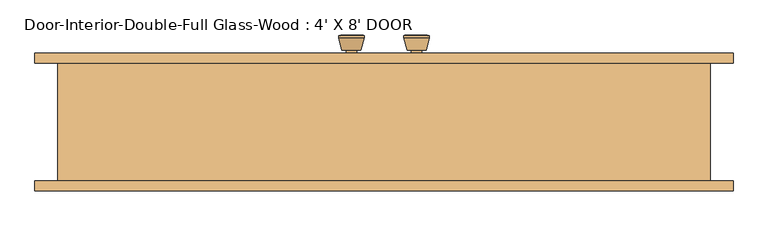
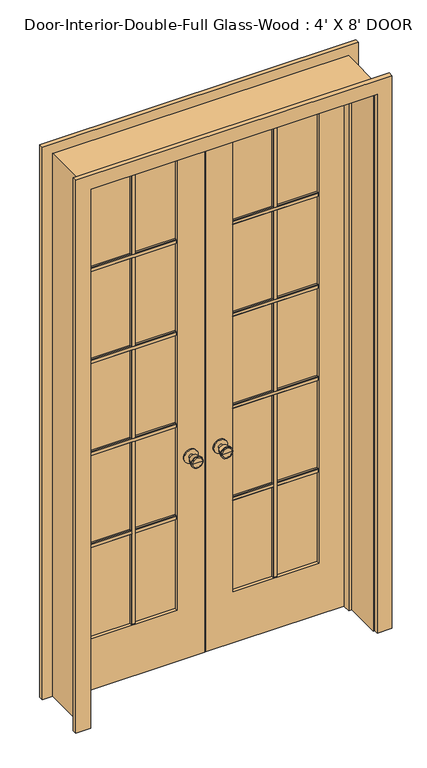
"""IFC4 building model written with IfcOpenShell, lengths in millimetres: door geometry, Door-Interior-Double-Full Glass-Wood : 4' X 8' DOOR."""

from ifc_helpers import new_model, si_unit, point, frame, frame_2d, origin, place, context, project, spatial, polyline, circle_curve, trimmed, segment, composite_curve, outline, extrude, faceted_brep, source, transform, mapped, element, save
from ifc_brep_helpers import plane_surface, cylinder_surface, revolved_surface, advanced_brep


def door_interior_double_full_glass_wood_4_x_8_door_7870f6d1(model_context):
    return source(origin(), model_context, "Body", "SolidModel", [
        advanced_brep(
        [(-63.5, 117.825, 914.4), (-73.5, 117.825, 914.4), (-53.5, 117.825, 914.4), (-83.9758676, 166.825, 914.4), (-63.5, 166.825, 914.4), (-43.0241324, 166.825, 914.4), (-88.5, 164.9971319, 914.4), (-38.5, 164.9971319, 914.4), (-88.5, 161.5334537, 914.4), (-38.5, 161.5334537, 914.4), (-82.136236, 136.825, 914.4), (-44.863764, 136.825, 914.4), (-73.5, 136.825, 914.4), (-53.5, 136.825, 914.4)],
        [
            (0, 1),
            (1, 2, circle_curve(frame((-63.5, 117.825, 914.4), z_axis=(0.0, -1.0, 0.0), x_axis=(1.0, 0.0, 0.0)), 10.0)),
            (2, 0),
            (2, 1, circle_curve(frame((-63.5, 117.825, 914.4), z_axis=(0.0, -1.0, 0.0), x_axis=(1.0, 0.0, 0.0)), 10.0)),
            (3, 4),
            (4, 5),
            (5, 3, circle_curve(frame((-63.5, 166.825, 914.4), z_axis=(0.0, 1.0, 0.0), x_axis=(1.0, 0.0, 0.0)), 20.4758676)),
            (3, 5, circle_curve(frame((-63.5, 166.825, 914.4), z_axis=(0.0, 1.0, 0.0), x_axis=(1.0, 0.0, 0.0)), 20.4758676)),
            (6, 3),
            (5, 7),
            (7, 6, circle_curve(frame((-63.5, 164.9971319, 914.4), z_axis=(0.0, 1.0, 0.0), x_axis=(1.0, 0.0, 0.0)), 25.0)),
            (6, 7, circle_curve(frame((-63.5, 164.9971319, 914.4), z_axis=(0.0, 1.0, 0.0), x_axis=(1.0, 0.0, 0.0)), 25.0)),
            (8, 6),
            (7, 9),
            (9, 8, circle_curve(frame((-63.5, 161.5334537, 914.4), z_axis=(0.0, 1.0, 0.0), x_axis=(1.0, 0.0, 0.0)), 25.0)),
            (8, 9, circle_curve(frame((-63.5, 161.5334537, 914.4), z_axis=(0.0, 1.0, 0.0), x_axis=(1.0, 0.0, 0.0)), 25.0)),
            (10, 8),
            (9, 11),
            (11, 10, circle_curve(frame((-63.5, 136.825, 914.4), z_axis=(0.0, 1.0, 0.0), x_axis=(1.0, 0.0, 0.0)), 18.636236)),
            (10, 11, circle_curve(frame((-63.5, 136.825, 914.4), z_axis=(0.0, 1.0, 0.0), x_axis=(1.0, 0.0, 0.0)), 18.636236)),
            (12, 10),
            (11, 13),
            (13, 12, circle_curve(frame((-63.5, 136.825, 914.4), z_axis=(0.0, 1.0, 0.0), x_axis=(1.0, 0.0, 0.0)), 10.0)),
            (12, 13, circle_curve(frame((-63.5, 136.825, 914.4), z_axis=(0.0, 1.0, 0.0), x_axis=(1.0, 0.0, 0.0)), 10.0)),
            (1, 12),
            (13, 2),
        ],
        [
            plane_surface(frame((-63.5, 117.825, 914.4), z_axis=(0.0, -1.0, 0.0), x_axis=(1.0, 0.0, 0.0))),
            plane_surface(frame((-63.5, 166.825, 914.4), z_axis=(0.0, 1.0, 0.0), x_axis=(1.0, 0.0, 0.0))),
            revolved_surface(polyline([(-43.0241324, 166.825, 914.4), (-38.5, 164.9971319, 914.4)]), (-63.5, 117.825, 914.4), (0.0, -1.0, 0.0)),
            cylinder_surface(frame((-63.5, 117.825, 914.4), z_axis=(0.0, -1.0, 0.0), x_axis=(1.0, 0.0, 0.0)), 25.0),
            revolved_surface(polyline([(-38.5, 161.5334537, 914.4), (-44.863764, 136.825, 914.4)]), (-63.5, 117.825, 914.4), (0.0, -1.0, 0.0)),
            plane_surface(frame((-63.5, 136.825, 914.4), z_axis=(0.0, -1.0, 0.0), x_axis=(1.0, 0.0, 0.0))),
            cylinder_surface(frame((-63.5, 117.825, 914.4), z_axis=(0.0, -1.0, 0.0), x_axis=(1.0, 0.0, 0.0)), 10.0),
        ],
        [
            (0, [[1, 2, 3]]),
            (0, [[-3, 4, -1]]),
            (1, [[5, 6, 7]]),
            (1, [[-6, -5, 8]]),
            (2, [[9, -7, 10, 11]]),
            (2, [[-10, -8, -9, 12]]),
            (3, [[13, -11, 14, 15]]),
            (3, [[-14, -12, -13, 16]]),
            (4, [[17, -15, 18, 19]]),
            (4, [[-18, -16, -17, 20]]),
            (5, [[21, -19, 22, 23]]),
            (5, [[-22, -20, -21, 24]]),
            (6, [[25, -23, 26, -2]]),
            (6, [[-26, -24, -25, -4]]),
        ],
    ),
        extrude(outline(composite_curve([segment(trimmed(circle_curve(frame_2d((914.4, -63.5)), 30.0), [point((914.4, -33.5))], [point((914.4, -93.5))], False, "CARTESIAN"), True, "CONTINUOUS"), segment(trimmed(circle_curve(frame_2d((914.4, -63.5)), 30.0), [point((914.4, -93.5))], [point((914.4, -33.5))], False, "CARTESIAN"), True, "CONTINUOUS")], self_intersect=False)), frame((0.0, 111.825, 0.0), z_axis=(0.0, 1.0, 0.0), x_axis=(0.0, 0.0, 1.0)), (0.0, 0.0, 1.0), 6.0),
        advanced_brep(
        [(-63.5, 70.9, 914.4), (-53.5, 70.9, 914.4), (-73.5, 70.9, 914.4), (-83.9758676, 21.9, 914.4), (-43.0241324, 21.9, 914.4), (-63.5, 21.9, 914.4), (-88.5, 23.7278681, 914.4), (-38.5, 23.7278681, 914.4), (-88.5, 27.1915463, 914.4), (-38.5, 27.1915463, 914.4), (-82.136236, 51.9, 914.4), (-44.863764, 51.9, 914.4), (-73.5, 51.9, 914.4), (-53.5, 51.9, 914.4)],
        [
            (0, 1),
            (1, 2, circle_curve(frame((-63.5, 70.9, 914.4), z_axis=(0.0, 1.0, 0.0), x_axis=(1.0, 0.0, 0.0)), 10.0)),
            (2, 0),
            (2, 1, circle_curve(frame((-63.5, 70.9, 914.4), z_axis=(0.0, 1.0, 0.0), x_axis=(1.0, 0.0, 0.0)), 10.0)),
            (3, 4, circle_curve(frame((-63.5, 21.9, 914.4), z_axis=(0.0, -1.0, 0.0), x_axis=(1.0, 0.0, 0.0)), 20.4758676)),
            (4, 5),
            (5, 3),
            (4, 3, circle_curve(frame((-63.5, 21.9, 914.4), z_axis=(0.0, -1.0, 0.0), x_axis=(1.0, 0.0, 0.0)), 20.4758676)),
            (6, 7, circle_curve(frame((-63.5, 23.7278681, 914.4), z_axis=(0.0, -1.0, 0.0), x_axis=(1.0, 0.0, 0.0)), 25.0)),
            (7, 4),
            (3, 6),
            (7, 6, circle_curve(frame((-63.5, 23.7278681, 914.4), z_axis=(0.0, -1.0, 0.0), x_axis=(1.0, 0.0, 0.0)), 25.0)),
            (8, 9, circle_curve(frame((-63.5, 27.1915463, 914.4), z_axis=(0.0, -1.0, 0.0), x_axis=(1.0, 0.0, 0.0)), 25.0)),
            (9, 7),
            (6, 8),
            (9, 8, circle_curve(frame((-63.5, 27.1915463, 914.4), z_axis=(0.0, -1.0, 0.0), x_axis=(1.0, 0.0, 0.0)), 25.0)),
            (10, 11, circle_curve(frame((-63.5, 51.9, 914.4), z_axis=(0.0, -1.0, 0.0), x_axis=(1.0, 0.0, 0.0)), 18.636236)),
            (11, 9),
            (8, 10),
            (11, 10, circle_curve(frame((-63.5, 51.9, 914.4), z_axis=(0.0, -1.0, 0.0), x_axis=(1.0, 0.0, 0.0)), 18.636236)),
            (12, 13, circle_curve(frame((-63.5, 51.9, 914.4), z_axis=(0.0, -1.0, 0.0), x_axis=(1.0, 0.0, 0.0)), 10.0)),
            (13, 11),
            (10, 12),
            (13, 12, circle_curve(frame((-63.5, 51.9, 914.4), z_axis=(0.0, -1.0, 0.0), x_axis=(1.0, 0.0, 0.0)), 10.0)),
            (1, 13),
            (12, 2),
        ],
        [
            plane_surface(frame((-63.5, 70.9, 914.4), z_axis=(0.0, 1.0, 0.0), x_axis=(1.0, 0.0, 0.0))),
            plane_surface(frame((-63.5, 21.9, 914.4), z_axis=(0.0, -1.0, 0.0), x_axis=(1.0, 0.0, 0.0))),
            revolved_surface(polyline([(-43.0241324, 21.9, 914.4), (-38.5, 23.7278681, 914.4)]), (-63.5, 70.9, 914.4), (0.0, 1.0, 0.0)),
            cylinder_surface(frame((-63.5, 70.9, 914.4), z_axis=(0.0, 1.0, 0.0), x_axis=(1.0, 0.0, 0.0)), 25.0),
            revolved_surface(polyline([(-38.5, 27.1915463, 914.4), (-44.863764, 51.9, 914.4)]), (-63.5, 70.9, 914.4), (0.0, 1.0, 0.0)),
            plane_surface(frame((-63.5, 51.9, 914.4), z_axis=(0.0, 1.0, 0.0), x_axis=(1.0, 0.0, 0.0))),
            cylinder_surface(frame((-63.5, 70.9, 914.4), z_axis=(0.0, 1.0, 0.0), x_axis=(1.0, 0.0, 0.0)), 10.0),
        ],
        [
            (0, [[1, 2, 3]]),
            (0, [[-3, 4, -1]]),
            (1, [[5, 6, 7]]),
            (1, [[8, -7, -6]]),
            (2, [[9, 10, -5, 11]]),
            (2, [[12, -11, -8, -10]]),
            (3, [[13, 14, -9, 15]]),
            (3, [[16, -15, -12, -14]]),
            (4, [[17, 18, -13, 19]]),
            (4, [[20, -19, -16, -18]]),
            (5, [[21, 22, -17, 23]]),
            (5, [[24, -23, -20, -22]]),
            (6, [[-2, 25, -21, 26]]),
            (6, [[-4, -26, -24, -25]]),
        ],
    ),
        extrude(outline(composite_curve([segment(trimmed(circle_curve(frame_2d((914.4, -63.5)), 30.0), [point((914.4, -33.5))], [point((914.4, -93.5))], False, "CARTESIAN"), True, "CONTINUOUS"), segment(trimmed(circle_curve(frame_2d((914.4, -63.5)), 30.0), [point((914.4, -93.5))], [point((914.4, -33.5))], False, "CARTESIAN"), True, "CONTINUOUS")], self_intersect=False)), frame((0.0, 70.9, 0.0), z_axis=(0.0, 1.0, 0.0), x_axis=(0.0, 0.0, 1.0)), (0.0, 0.0, 1.0), 6.0),
        extrude(outline(polyline([(90.87, 1911.35), (90.87, 1892.3), (84.52, 1892.3), (81.345, 1895.475), (81.345, 1908.175), (84.52, 1911.35), (90.87, 1911.35)])), frame((120.65, 0.0, 0.0), z_axis=(1.0, 0.0, 0.0), x_axis=(0.0, 1.0, 0.0)), (0.0, 0.0, 1.0), 368.3),
        extrude(outline(polyline([(90.87, 1493.8375), (90.87, 1474.7875), (84.52, 1474.7875), (81.345, 1477.9625), (81.345, 1490.6625), (84.52, 1493.8375), (90.87, 1493.8375)])), frame((120.65, 0.0, 0.0), z_axis=(1.0, 0.0, 0.0), x_axis=(0.0, 1.0, 0.0)), (0.0, 0.0, 1.0), 368.3),
        extrude(outline(polyline([(90.87, 1076.325), (90.87, 1057.275), (84.52, 1057.275), (81.345, 1060.45), (81.345, 1073.15), (84.52, 1076.325), (90.87, 1076.325)])), frame((120.65, 0.0, 0.0), z_axis=(1.0, 0.0, 0.0), x_axis=(0.0, 1.0, 0.0)), (0.0, 0.0, 1.0), 368.3),
        extrude(outline(polyline([(295.275, 90.87), (314.325, 90.87), (314.325, 84.52), (311.15, 81.345), (298.45, 81.345), (295.275, 84.52), (295.275, 90.87)])), frame((0.0, 0.0, 231.775), z_axis=(0.0, 0.0, 1.0), x_axis=(1.0, 0.0, 0.0)), (0.0, 0.0, 1.0), 2087.5625),
        extrude(outline(polyline([(90.87, 658.8125), (90.87, 639.7625), (84.52, 639.7625), (81.345, 642.9375), (81.345, 655.6375), (84.52, 658.8125), (90.87, 658.8125)])), frame((120.65, 0.0, 0.0), z_axis=(1.0, 0.0, 0.0), x_axis=(0.0, 1.0, 0.0)), (0.0, 0.0, 1.0), 368.3),
        extrude(outline(polyline([(97.855, 1911.35), (104.205, 1911.35), (107.38, 1908.175), (107.38, 1895.475), (104.205, 1892.3), (97.855, 1892.3), (97.855, 1911.35)])), frame((-488.95, 0.0, 0.0), z_axis=(1.0, 0.0, 0.0), x_axis=(0.0, 1.0, 0.0)), (0.0, 0.0, 1.0), 368.3),
        extrude(outline(polyline([(97.855, 1493.8375), (104.205, 1493.8375), (107.38, 1490.6625), (107.38, 1477.9625), (104.205, 1474.7875), (97.855, 1474.7875), (97.855, 1493.8375)])), frame((-488.95, 0.0, 0.0), z_axis=(1.0, 0.0, 0.0), x_axis=(0.0, 1.0, 0.0)), (0.0, 0.0, 1.0), 368.3),
        extrude(outline(polyline([(97.855, 1076.325), (104.205, 1076.325), (107.38, 1073.15), (107.38, 1060.45), (104.205, 1057.275), (97.855, 1057.275), (97.855, 1076.325)])), frame((-488.95, 0.0, 0.0), z_axis=(1.0, 0.0, 0.0), x_axis=(0.0, 1.0, 0.0)), (0.0, 0.0, 1.0), 368.3),
        extrude(outline(polyline([(-314.325, 97.855), (-314.325, 104.205), (-311.15, 107.38), (-298.45, 107.38), (-295.275, 104.205), (-295.275, 97.855), (-314.325, 97.855)])), frame((0.0, 0.0, 231.775), z_axis=(0.0, 0.0, 1.0), x_axis=(1.0, 0.0, 0.0)), (0.0, 0.0, 1.0), 2087.5625),
        extrude(outline(polyline([(97.855, 658.8125), (104.205, 658.8125), (107.38, 655.6375), (107.38, 642.9375), (104.205, 639.7625), (97.855, 639.7625), (97.855, 658.8125)])), frame((-488.95, 0.0, 0.0), z_axis=(1.0, 0.0, 0.0), x_axis=(0.0, 1.0, 0.0)), (0.0, 0.0, 1.0), 368.3),
        extrude(outline(polyline([(97.855, 1911.35), (104.205, 1911.35), (107.38, 1908.175), (107.38, 1895.475), (104.205, 1892.3), (97.855, 1892.3), (97.855, 1911.35)])), frame((120.65, 0.0, 0.0), z_axis=(1.0, 0.0, 0.0), x_axis=(0.0, 1.0, 0.0)), (0.0, 0.0, 1.0), 368.3),
        extrude(outline(polyline([(97.855, 1493.8375), (104.205, 1493.8375), (107.38, 1490.6625), (107.38, 1477.9625), (104.205, 1474.7875), (97.855, 1474.7875), (97.855, 1493.8375)])), frame((120.65, 0.0, 0.0), z_axis=(1.0, 0.0, 0.0), x_axis=(0.0, 1.0, 0.0)), (0.0, 0.0, 1.0), 368.3),
        extrude(outline(polyline([(97.855, 1076.325), (104.205, 1076.325), (107.38, 1073.15), (107.38, 1060.45), (104.205, 1057.275), (97.855, 1057.275), (97.855, 1076.325)])), frame((120.65, 0.0, 0.0), z_axis=(1.0, 0.0, 0.0), x_axis=(0.0, 1.0, 0.0)), (0.0, 0.0, 1.0), 368.3),
        extrude(outline(polyline([(295.275, 97.855), (295.275, 104.205), (298.45, 107.38), (311.15, 107.38), (314.325, 104.205), (314.325, 97.855), (295.275, 97.855)])), frame((0.0, 0.0, 231.775), z_axis=(0.0, 0.0, 1.0), x_axis=(1.0, 0.0, 0.0)), (0.0, 0.0, 1.0), 2087.5625),
        extrude(outline(polyline([(97.855, 658.8125), (104.205, 658.8125), (107.38, 655.6375), (107.38, 642.9375), (104.205, 639.7625), (97.855, 639.7625), (97.855, 658.8125)])), frame((120.65, 0.0, 0.0), z_axis=(1.0, 0.0, 0.0), x_axis=(0.0, 1.0, 0.0)), (0.0, 0.0, 1.0), 368.3),
        extrude(outline(polyline([(90.87, 1911.35), (90.87, 1892.3), (84.52, 1892.3), (81.345, 1895.475), (81.345, 1908.175), (84.52, 1911.35), (90.87, 1911.35)])), frame((-488.95, 0.0, 0.0), z_axis=(1.0, 0.0, 0.0), x_axis=(0.0, 1.0, 0.0)), (0.0, 0.0, 1.0), 368.3),
        extrude(outline(polyline([(90.87, 1493.8375), (90.87, 1474.7875), (84.52, 1474.7875), (81.345, 1477.9625), (81.345, 1490.6625), (84.52, 1493.8375), (90.87, 1493.8375)])), frame((-488.95, 0.0, 0.0), z_axis=(1.0, 0.0, 0.0), x_axis=(0.0, 1.0, 0.0)), (0.0, 0.0, 1.0), 368.3),
        extrude(outline(polyline([(90.87, 1076.325), (90.87, 1057.275), (84.52, 1057.275), (81.345, 1060.45), (81.345, 1073.15), (84.52, 1076.325), (90.87, 1076.325)])), frame((-488.95, 0.0, 0.0), z_axis=(1.0, 0.0, 0.0), x_axis=(0.0, 1.0, 0.0)), (0.0, 0.0, 1.0), 368.3),
        extrude(outline(polyline([(-314.325, 90.87), (-295.275, 90.87), (-295.275, 84.52), (-298.45, 81.345), (-311.15, 81.345), (-314.325, 84.52), (-314.325, 90.87)])), frame((0.0, 0.0, 231.775), z_axis=(0.0, 0.0, 1.0), x_axis=(1.0, 0.0, 0.0)), (0.0, 0.0, 1.0), 2087.5625),
        extrude(outline(polyline([(90.87, 658.8125), (90.87, 639.7625), (84.52, 639.7625), (81.345, 642.9375), (81.345, 655.6375), (84.52, 658.8125), (90.87, 658.8125)])), frame((-488.95, 0.0, 0.0), z_axis=(1.0, 0.0, 0.0), x_axis=(0.0, 1.0, 0.0)), (0.0, 0.0, 1.0), 368.3),
        advanced_brep(
        [(63.5, 70.9, 914.4), (73.5, 70.9, 914.4), (53.5, 70.9, 914.4), (83.9758676, 21.9, 914.4), (63.5, 21.9, 914.4), (43.0241324, 21.9, 914.4), (88.5, 23.7278681, 914.4), (38.5, 23.7278681, 914.4), (88.5, 27.1915463, 914.4), (38.5, 27.1915463, 914.4), (82.136236, 51.9, 914.4), (44.863764, 51.9, 914.4), (73.5, 51.9, 914.4), (53.5, 51.9, 914.4)],
        [
            (0, 1),
            (1, 2, circle_curve(frame((63.5, 70.9, 914.4), z_axis=(0.0, 1.0, 0.0), x_axis=(-1.0, 0.0, 0.0)), 10.0)),
            (2, 0),
            (2, 1, circle_curve(frame((63.5, 70.9, 914.4), z_axis=(0.0, 1.0, 0.0), x_axis=(-1.0, 0.0, 0.0)), 10.0)),
            (3, 4),
            (4, 5),
            (5, 3, circle_curve(frame((63.5, 21.9, 914.4), z_axis=(0.0, -1.0, 0.0), x_axis=(-1.0, 0.0, 0.0)), 20.4758676)),
            (3, 5, circle_curve(frame((63.5, 21.9, 914.4), z_axis=(0.0, -1.0, 0.0), x_axis=(-1.0, 0.0, 0.0)), 20.4758676)),
            (6, 3),
            (5, 7),
            (7, 6, circle_curve(frame((63.5, 23.7278681, 914.4), z_axis=(0.0, -1.0, 0.0), x_axis=(-1.0, 0.0, 0.0)), 25.0)),
            (6, 7, circle_curve(frame((63.5, 23.7278681, 914.4), z_axis=(0.0, -1.0, 0.0), x_axis=(-1.0, 0.0, 0.0)), 25.0)),
            (8, 6),
            (7, 9),
            (9, 8, circle_curve(frame((63.5, 27.1915463, 914.4), z_axis=(0.0, -1.0, 0.0), x_axis=(-1.0, 0.0, 0.0)), 25.0)),
            (8, 9, circle_curve(frame((63.5, 27.1915463, 914.4), z_axis=(0.0, -1.0, 0.0), x_axis=(-1.0, 0.0, 0.0)), 25.0)),
            (10, 8),
            (9, 11),
            (11, 10, circle_curve(frame((63.5, 51.9, 914.4), z_axis=(0.0, -1.0, 0.0), x_axis=(-1.0, 0.0, 0.0)), 18.636236)),
            (10, 11, circle_curve(frame((63.5, 51.9, 914.4), z_axis=(0.0, -1.0, 0.0), x_axis=(-1.0, 0.0, 0.0)), 18.636236)),
            (12, 10),
            (11, 13),
            (13, 12, circle_curve(frame((63.5, 51.9, 914.4), z_axis=(0.0, -1.0, 0.0), x_axis=(-1.0, 0.0, 0.0)), 10.0)),
            (12, 13, circle_curve(frame((63.5, 51.9, 914.4), z_axis=(0.0, -1.0, 0.0), x_axis=(-1.0, 0.0, 0.0)), 10.0)),
            (1, 12),
            (13, 2),
        ],
        [
            plane_surface(frame((63.5, 70.9, 914.4), z_axis=(0.0, 1.0, 0.0), x_axis=(-1.0, 0.0, 0.0))),
            plane_surface(frame((63.5, 21.9, 914.4), z_axis=(0.0, -1.0, 0.0), x_axis=(-1.0, 0.0, 0.0))),
            revolved_surface(polyline([(43.0241324, 21.9, 914.4), (38.5, 23.7278681, 914.4)]), (63.5, 70.9, 914.4), (0.0, 1.0, 0.0)),
            cylinder_surface(frame((63.5, 70.9, 914.4), z_axis=(0.0, 1.0, 0.0), x_axis=(-1.0, 0.0, 0.0)), 25.0),
            revolved_surface(polyline([(38.5, 27.1915463, 914.4), (44.863764, 51.9, 914.4)]), (63.5, 70.9, 914.4), (0.0, 1.0, 0.0)),
            plane_surface(frame((63.5, 51.9, 914.4), z_axis=(0.0, 1.0, 0.0), x_axis=(-1.0, 0.0, 0.0))),
            cylinder_surface(frame((63.5, 70.9, 914.4), z_axis=(0.0, 1.0, 0.0), x_axis=(-1.0, 0.0, 0.0)), 10.0),
        ],
        [
            (0, [[1, 2, 3]]),
            (0, [[-3, 4, -1]]),
            (1, [[5, 6, 7]]),
            (1, [[-6, -5, 8]]),
            (2, [[9, -7, 10, 11]]),
            (2, [[-10, -8, -9, 12]]),
            (3, [[13, -11, 14, 15]]),
            (3, [[-14, -12, -13, 16]]),
            (4, [[17, -15, 18, 19]]),
            (4, [[-18, -16, -17, 20]]),
            (5, [[21, -19, 22, 23]]),
            (5, [[-22, -20, -21, 24]]),
            (6, [[25, -23, 26, -2]]),
            (6, [[-26, -24, -25, -4]]),
        ],
    ),
        extrude(outline(composite_curve([segment(trimmed(circle_curve(frame_2d((914.4, 63.5)), 30.0), [point((914.4, 33.5))], [point((914.4, 93.5))], False, "CARTESIAN"), True, "CONTINUOUS"), segment(trimmed(circle_curve(frame_2d((914.4, 63.5)), 30.0), [point((914.4, 93.5))], [point((914.4, 33.5))], False, "CARTESIAN"), True, "CONTINUOUS")], self_intersect=False)), frame((0.0, 70.9, 0.0), z_axis=(0.0, 1.0, 0.0), x_axis=(0.0, 0.0, 1.0)), (0.0, 0.0, 1.0), 6.0),
        advanced_brep(
        [(63.5, 117.825, 914.4), (53.5, 117.825, 914.4), (73.5, 117.825, 914.4), (83.9758676, 166.825, 914.4), (43.0241324, 166.825, 914.4), (63.5, 166.825, 914.4), (88.5, 164.9971319, 914.4), (38.5, 164.9971319, 914.4), (88.5, 161.5334537, 914.4), (38.5, 161.5334537, 914.4), (82.136236, 136.825, 914.4), (44.863764, 136.825, 914.4), (73.5, 136.825, 914.4), (53.5, 136.825, 914.4)],
        [
            (0, 1),
            (1, 2, circle_curve(frame((63.5, 117.825, 914.4), z_axis=(0.0, -1.0, 0.0), x_axis=(-1.0, 0.0, 0.0)), 10.0)),
            (2, 0),
            (2, 1, circle_curve(frame((63.5, 117.825, 914.4), z_axis=(0.0, -1.0, 0.0), x_axis=(-1.0, 0.0, 0.0)), 10.0)),
            (3, 4, circle_curve(frame((63.5, 166.825, 914.4), z_axis=(0.0, 1.0, 0.0), x_axis=(-1.0, 0.0, 0.0)), 20.4758676)),
            (4, 5),
            (5, 3),
            (4, 3, circle_curve(frame((63.5, 166.825, 914.4), z_axis=(0.0, 1.0, 0.0), x_axis=(-1.0, 0.0, 0.0)), 20.4758676)),
            (6, 7, circle_curve(frame((63.5, 164.9971319, 914.4), z_axis=(0.0, 1.0, 0.0), x_axis=(-1.0, 0.0, 0.0)), 25.0)),
            (7, 4),
            (3, 6),
            (7, 6, circle_curve(frame((63.5, 164.9971319, 914.4), z_axis=(0.0, 1.0, 0.0), x_axis=(-1.0, 0.0, 0.0)), 25.0)),
            (8, 9, circle_curve(frame((63.5, 161.5334537, 914.4), z_axis=(0.0, 1.0, 0.0), x_axis=(-1.0, 0.0, 0.0)), 25.0)),
            (9, 7),
            (6, 8),
            (9, 8, circle_curve(frame((63.5, 161.5334537, 914.4), z_axis=(0.0, 1.0, 0.0), x_axis=(-1.0, 0.0, 0.0)), 25.0)),
            (10, 11, circle_curve(frame((63.5, 136.825, 914.4), z_axis=(0.0, 1.0, 0.0), x_axis=(-1.0, 0.0, 0.0)), 18.636236)),
            (11, 9),
            (8, 10),
            (11, 10, circle_curve(frame((63.5, 136.825, 914.4), z_axis=(0.0, 1.0, 0.0), x_axis=(-1.0, 0.0, 0.0)), 18.636236)),
            (12, 13, circle_curve(frame((63.5, 136.825, 914.4), z_axis=(0.0, 1.0, 0.0), x_axis=(-1.0, 0.0, 0.0)), 10.0)),
            (13, 11),
            (10, 12),
            (13, 12, circle_curve(frame((63.5, 136.825, 914.4), z_axis=(0.0, 1.0, 0.0), x_axis=(-1.0, 0.0, 0.0)), 10.0)),
            (1, 13),
            (12, 2),
        ],
        [
            plane_surface(frame((63.5, 117.825, 914.4), z_axis=(0.0, -1.0, 0.0), x_axis=(-1.0, 0.0, 0.0))),
            plane_surface(frame((63.5, 166.825, 914.4), z_axis=(0.0, 1.0, 0.0), x_axis=(-1.0, 0.0, 0.0))),
            revolved_surface(polyline([(43.0241324, 166.825, 914.4), (38.5, 164.9971319, 914.4)]), (63.5, 117.825, 914.4), (0.0, -1.0, 0.0)),
            cylinder_surface(frame((63.5, 117.825, 914.4), z_axis=(0.0, -1.0, 0.0), x_axis=(-1.0, 0.0, 0.0)), 25.0),
            revolved_surface(polyline([(38.5, 161.5334537, 914.4), (44.863764, 136.825, 914.4)]), (63.5, 117.825, 914.4), (0.0, -1.0, 0.0)),
            plane_surface(frame((63.5, 136.825, 914.4), z_axis=(0.0, -1.0, 0.0), x_axis=(-1.0, 0.0, 0.0))),
            cylinder_surface(frame((63.5, 117.825, 914.4), z_axis=(0.0, -1.0, 0.0), x_axis=(-1.0, 0.0, 0.0)), 10.0),
        ],
        [
            (0, [[1, 2, 3]]),
            (0, [[-3, 4, -1]]),
            (1, [[5, 6, 7]]),
            (1, [[8, -7, -6]]),
            (2, [[9, 10, -5, 11]]),
            (2, [[12, -11, -8, -10]]),
            (3, [[13, 14, -9, 15]]),
            (3, [[16, -15, -12, -14]]),
            (4, [[17, 18, -13, 19]]),
            (4, [[20, -19, -16, -18]]),
            (5, [[21, 22, -17, 23]]),
            (5, [[24, -23, -20, -22]]),
            (6, [[-2, 25, -21, 26]]),
            (6, [[-4, -26, -24, -25]]),
        ],
    ),
        extrude(outline(composite_curve([segment(trimmed(circle_curve(frame_2d((914.4, 63.5)), 30.0), [point((914.4, 33.5))], [point((914.4, 93.5))], False, "CARTESIAN"), True, "CONTINUOUS"), segment(trimmed(circle_curve(frame_2d((914.4, 63.5)), 30.0), [point((914.4, 93.5))], [point((914.4, 33.5))], False, "CARTESIAN"), True, "CONTINUOUS")], self_intersect=False)), frame((0.0, 111.825, 0.0), z_axis=(0.0, 1.0, 0.0), x_axis=(0.0, 0.0, 1.0)), (0.0, 0.0, 1.0), 6.0),
        extrude(outline(polyline([(0.0, 615.95), (0.0, 679.45), (2508.25, 679.45), (2508.25, -679.45), (0.0, -679.45), (0.0, -615.95), (2444.75, -615.95), (2444.75, 615.95), (0.0, 615.95)])), frame((0.0, -137.225, 0.0), z_axis=(0.0, 1.0, 0.0), x_axis=(0.0, 0.0, 1.0)), (0.0, 0.0, 1.0), 19.05),
        extrude(outline(polyline([(0.0, 615.95), (0.0, 679.45), (2508.25, 679.45), (2508.25, -679.45), (0.0, -679.45), (0.0, -615.95), (2444.75, -615.95), (2444.75, 615.95), (0.0, 615.95)])), frame((0.0, 111.825, 0.0), z_axis=(0.0, 1.0, 0.0), x_axis=(0.0, 0.0, 1.0)), (0.0, 0.0, 1.0), 19.05),
        faceted_brep([(635.0, 111.825, 0.0), (635.0, -118.175, 0.0), (609.6, -118.175, 0.0), (609.6, 41.975, 0.0), (596.9, 41.975, 0.0), (596.9, 76.9, 0.0), (609.6, 76.9, 0.0), (609.6, 111.825, 0.0), (635.0, 111.825, 2463.8), (635.0, -118.175, 2463.8), (-635.0, -118.175, 2463.8), (-635.0, -118.175, 0.0), (-609.6, -118.175, 0.0), (-609.6, -118.175, 2438.4), (609.6, -118.175, 2438.4), (609.6, 41.975, 2438.4), (-609.6, 41.975, 2438.4), (-609.6, 41.975, 0.0), (-596.9, 41.975, 0.0), (-596.9, 41.975, 2425.7), (596.9, 41.975, 2425.7), (596.9, 76.9, 2425.7), (1.5875, 76.9, 2425.7), (-1.6019111, 76.9, 2425.7), (-596.9, 76.9, 2425.7), (-596.9, 76.9, 0.0), (-609.6, 76.9, 0.0), (-609.6, 76.9, 2438.4), (-1.6019111, 76.9, 2438.4), (1.5875, 76.9, 2438.4), (609.6, 76.9, 2438.4), (609.6, 111.825, 2438.4), (1.5875, 111.825, 2438.4), (-1.6019111, 111.825, 2438.4), (-609.6, 111.825, 2438.4), (-609.6, 111.825, 0.0), (-635.0, 111.825, 0.0), (-635.0, 111.825, 2463.8)], [[[0, 1, 2, 3, 4, 5, 6, 7]], [[1, 0, 8, 9]], [[2, 1, 9, 10, 11, 12, 13, 14]], [[3, 2, 14, 15]], [[4, 3, 15, 16, 17, 18, 19, 20]], [[5, 4, 20, 21]], [[6, 5, 21, 22, 23, 24, 25, 26, 27, 28, 29, 30]], [[7, 6, 30, 31]], [[0, 7, 31, 32, 33, 34, 35, 36, 37, 8]], [[9, 8, 37, 10]], [[14, 13, 16, 15]], [[20, 19, 24, 23, 22, 21]], [[31, 30, 29, 28, 27, 34, 33, 32]], [[12, 11, 36, 35, 26, 25, 18, 17]], [[11, 10, 37, 36]], [[13, 12, 17, 16]], [[19, 18, 25, 24]], [[27, 26, 35, 34]]]),
        extrude(outline(polyline([(2438.4, -609.6), (0.0, -609.6), (0.0, -1.6019111), (2438.4, -1.6019111), (2438.4, -609.6)]), holes=[polyline([(231.775, -488.95), (2319.3375, -488.95), (2319.3375, -120.65), (231.775, -120.65), (231.775, -488.95)])]), frame((0.0, 76.9, 0.0), z_axis=(0.0, 1.0, 0.0), x_axis=(0.0, 0.0, 1.0)), (0.0, 0.0, 1.0), 34.925),
        extrude(outline(polyline([(0.0, 609.6), (2438.4, 609.6), (2438.4, 1.5875), (0.0, 1.5875), (0.0, 609.6)]), holes=[polyline([(2319.3375, 120.65), (2319.3375, 488.95), (231.775, 488.95), (231.775, 120.65), (2319.3375, 120.65)])]), frame((0.0, 76.9, 0.0), z_axis=(0.0, 1.0, 0.0), x_axis=(0.0, 0.0, 1.0)), (0.0, 0.0, 1.0), 34.925),
        extrude(outline(polyline([(488.95, 90.87), (120.65, 90.87), (120.65, 97.855), (488.95, 97.855), (488.95, 90.87)])), frame((0.0, 0.0, 231.775), z_axis=(0.0, 0.0, 1.0), x_axis=(1.0, 0.0, 0.0)), (0.0, 0.0, 1.0), 2087.5625),
        extrude(outline(polyline([(-120.65, 90.87), (-488.95, 90.87), (-488.95, 97.855), (-120.65, 97.855), (-120.65, 90.87)])), frame((0.0, 0.0, 231.775), z_axis=(0.0, 0.0, 1.0), x_axis=(1.0, 0.0, 0.0)), (0.0, 0.0, 1.0), 2087.5625),
    ])


if __name__ == "__main__":
    model = new_model("IFC4")
    model_context = context("Model", 3, world=origin())
    ifc_project = project(units=[si_unit("LENGTHUNIT", "METRE", prefix="MILLI")], contexts=[model_context])
    site = spatial("IfcSite", under=ifc_project)
    building = spatial("IfcBuilding", under=site)
    placement = place(None, origin())
    door_interior_double_full_glass_wood_4_x_8_door_shape = door_interior_double_full_glass_wood_4_x_8_door_7870f6d1(model_context)
    element("IfcDoor", 1, ObjectType="Door-Interior-Double-Full Glass-Wood : 4' X 8' DOOR", at=placement, inside=building, context=model_context, shape_type="MappedRepresentation", body=[
        mapped(door_interior_double_full_glass_wood_4_x_8_door_shape, transform((0.0, 0.0, 0.0), x_axis=(1.0, 0.0, 0.0), y_axis=(0.0, 1.0, 0.0), z_axis=(0.0, 0.0, 1.0))),
    ])
    save(model, "model.ifc")

# Revit data of these elements
# Type "Door-Interior-Double-Full Glass-Wood : 4' X 8' DOOR"
#   Type Mark = "12"
#   Assembly Code = "C1020300"
#   Analytic Construction = "French door, wood frame with single glass"
#   Top Rail = 0' - 4 11/16"
#   Thickness = 0' - 1 3/8"
#   Thermal Resistance (R) = 1.0696 (h·ft²·°F)/BTU
#   Swing Angle [instance default] = 90.00°
#   Stiles = 0' - 4 3/4"
#   Rough Width = 4' - 2"
#   Rough Height = 8' - 1"
#   Panel Width = 2' - 0"
#   Height = 8' - 0"
#   Width = 4' - 0"
#   Heat Transfer Coefficient (U) = 0.9350 BTU/(h·ft²·°F)
#   Bottom Rail = 0' - 9 1/8"
#   Show Grill [instance default] = yes
#   Trim Material = Cherry
#   Panel Material = Cherry
#   Frame Material = Cherry
#   Door Handle Material = Aluminum
#   Visual Light Transmittance = 0
#   Solar Heat Gain Coefficient = 0
#   Wall Closure = (empty or 0)
#   Function = (empty or 0)
# Element 1 (IfcDoor, "Door-Interior-Double-Full Glass-Wood : 4' X 8' DOOR")
#   Materials on its faces: "Cherry", "Aluminum", "Glass"
# Materials
#   "Cherry": class "Wood", colour RGB 226 177 128, transparency 0, Description = "Prunus Serotina", Cost = 0
#   "Aluminum": class "Metal", colour RGB 247 247 247, transparency 0, Description = "Aluminum 6061", Cost = 0
#   "Glass": class "Glass", colour RGB 0 128 192, transparency 0.75, Description = "Soda Lime Glass", Cost = 0
